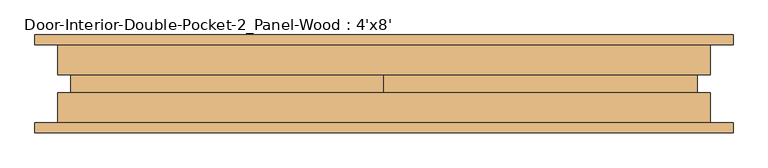
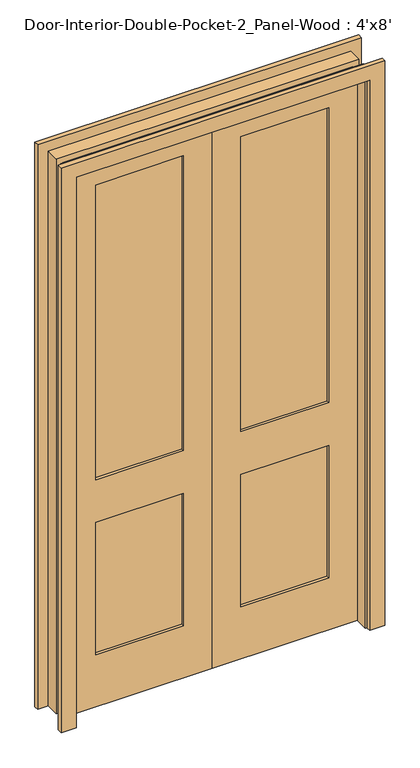
"""IFC4 building model written with IfcOpenShell, lengths in millimetres: door geometry, Door-Interior-Double-Pocket-2_Panel-Wood : 4'x8'."""

from ifc_helpers import new_model, si_unit, frame, origin, place, context, project, spatial, polyline, outline, extrude, source, transform, mapped, element, save


def door_interior_double_pocket_2_panel_wood_4_x8_0aea24c3(model_context):
    return source(origin(), model_context, "Body", "SweptSolid", [
        extrude(outline(polyline([(0.0, 615.95), (0.0, 679.45), (2508.25, 679.45), (2508.25, -679.45), (0.0, -679.45), (0.0, -615.95), (2444.75, -615.95), (2444.75, 615.95), (0.0, 615.95)])), frame((0.0, 76.2, 0.0), z_axis=(0.0, 1.0, 0.0), x_axis=(0.0, 0.0, 1.0)), (0.0, 0.0, 1.0), 19.05),
        extrude(outline(polyline([(0.0, 615.95), (0.0, 679.45), (2508.25, 679.45), (2508.25, -679.45), (0.0, -679.45), (0.0, -615.95), (2444.75, -615.95), (2444.75, 615.95), (0.0, 615.95)])), frame((0.0, -95.25, 0.0), z_axis=(0.0, 1.0, 0.0), x_axis=(0.0, 0.0, 1.0)), (0.0, 0.0, 1.0), 19.05),
        extrude(outline(polyline([(2438.4, 0.0), (0.0, 0.0), (0.0, 609.6), (2438.4, 609.6), (2438.4, 0.0)]), holes=[polyline([(2319.3375, 120.65), (2319.3375, 488.95), (1009.65, 488.95), (1009.65, 120.65), (2319.3375, 120.65)]), polyline([(819.15, 120.65), (819.15, 488.95), (231.775, 488.95), (231.775, 120.65), (819.15, 120.65)])]), frame((0.0, -17.4625, 0.0), z_axis=(0.0, 1.0, 0.0), x_axis=(0.0, 0.0, 1.0)), (0.0, 0.0, 1.0), 34.925),
        extrude(outline(polyline([(488.95, -5.8208333), (120.65, -5.8208333), (120.65, 5.8208333), (488.95, 5.8208333), (488.95, -5.8208333)])), frame((0.0, 0.0, 1009.65), z_axis=(0.0, 0.0, 1.0), x_axis=(1.0, 0.0, 0.0)), (0.0, 0.0, 1.0), 1309.6875),
        extrude(outline(polyline([(488.95, -5.8208333), (120.65, -5.8208333), (120.65, 5.8208333), (488.95, 5.8208333), (488.95, -5.8208333)])), frame((0.0, 0.0, 231.775), z_axis=(0.0, 0.0, 1.0), x_axis=(1.0, 0.0, 0.0)), (0.0, 0.0, 1.0), 587.375),
        extrude(outline(polyline([(0.0, 635.0), (2463.8, 635.0), (2463.8, -635.0), (0.0, -635.0), (0.0, -609.6), (2438.4, -609.6), (2438.4, 609.6), (0.0, 609.6), (0.0, 635.0)])), frame((0.0, 17.4625, 0.0), z_axis=(0.0, 1.0, 0.0), x_axis=(0.0, 0.0, 1.0)), (0.0, 0.0, 1.0), 58.7375),
        extrude(outline(polyline([(0.0, 635.0), (2463.8, 635.0), (2463.8, -635.0), (0.0, -635.0), (0.0, -609.6), (2438.4, -609.6), (2438.4, 609.6), (0.0, 609.6), (0.0, 635.0)])), frame((0.0, -76.2, 0.0), z_axis=(0.0, 1.0, 0.0), x_axis=(0.0, 0.0, 1.0)), (0.0, 0.0, 1.0), 58.7375),
        extrude(outline(polyline([(2438.4, -609.6), (0.0, -609.6), (0.0, 0.0), (2438.4, 0.0), (2438.4, -609.6)]), holes=[polyline([(2319.3375, -488.95), (2319.3375, -120.65), (1009.65, -120.65), (1009.65, -488.95), (2319.3375, -488.95)]), polyline([(819.15, -488.95), (819.15, -120.65), (231.775, -120.65), (231.775, -488.95), (819.15, -488.95)])]), frame((0.0, -17.4625, 0.0), z_axis=(0.0, 1.0, 0.0), x_axis=(0.0, 0.0, 1.0)), (0.0, 0.0, 1.0), 34.925),
        extrude(outline(polyline([(-120.65, -5.8208333), (-488.95, -5.8208333), (-488.95, 5.8208333), (-120.65, 5.8208333), (-120.65, -5.8208333)])), frame((0.0, 0.0, 1009.65), z_axis=(0.0, 0.0, 1.0), x_axis=(1.0, 0.0, 0.0)), (0.0, 0.0, 1.0), 1309.6875),
        extrude(outline(polyline([(-120.65, -5.8208333), (-488.95, -5.8208333), (-488.95, 5.8208333), (-120.65, 5.8208333), (-120.65, -5.8208333)])), frame((0.0, 0.0, 231.775), z_axis=(0.0, 0.0, 1.0), x_axis=(1.0, 0.0, 0.0)), (0.0, 0.0, 1.0), 587.375),
    ])


if __name__ == "__main__":
    model = new_model("IFC4")
    model_context = context("Model", 3, world=origin())
    ifc_project = project(units=[si_unit("LENGTHUNIT", "METRE", prefix="MILLI")], contexts=[model_context])
    site = spatial("IfcSite", under=ifc_project)
    building = spatial("IfcBuilding", under=site)
    placement = place(None, origin())
    door_interior_double_pocket_2_panel_wood_4_x8_shape = door_interior_double_pocket_2_panel_wood_4_x8_0aea24c3(model_context)
    element("IfcDoor", 1, ObjectType="Door-Interior-Double-Pocket-2_Panel-Wood : 4'x8'", at=placement, inside=building, context=model_context, shape_type="MappedRepresentation", body=[
        mapped(door_interior_double_pocket_2_panel_wood_4_x8_shape, transform((0.0, 0.0, 0.0), x_axis=(1.0, 0.0, 0.0), y_axis=(0.0, 1.0, 0.0), z_axis=(0.0, 0.0, 1.0))),
    ])
    save(model, "model.ifc")

# Revit data of these elements
# Type "Door-Interior-Double-Pocket-2_Panel-Wood : 4'x8'"
#   Type Mark = "11"
#   Assembly Code = "C1020300"
#   Analytic Construction = "Wooden"
#   Top Rail = 0' - 4 11/16"
#   Thickness = 0' - 1 3/8"
#   Thermal Resistance (R) = 2.5876 (h·ft²·°F)/BTU
#   Stiles = 0' - 4 3/4"
#   Rough Width = 8' - 2"
#   Rough Height = 8' - 4 1/2"
#   Panel Width = 2' - 0"
#   Lock Rail = 0' - 7 1/2"
#   Location [instance default] = 2' - 1"
#   Height = 8' - 0"
#   Width = 4' - 0"
#   Heat Transfer Coefficient (U) = 0.3865 BTU/(h·ft²·°F)
#   Bottom Rail = 0' - 9 1/8"
#   Panel Open [instance default] = no
#   Trim Material = Cherry
#   Panel Material = Cherry
#   Frame Material = Cherry
#   Visual Light Transmittance = 0
#   Solar Heat Gain Coefficient = 0
#   Wall Closure = (empty or 0)
#   Function = (empty or 0)
# Element 1 (IfcDoor, "Door-Interior-Double-Pocket-2_Panel-Wood : 4'x8'")
#   Materials on its faces: "Cherry"
# Materials
#   "Cherry": class "Wood", colour RGB 226 177 128, transparency 0, Description = "Prunus Serotina", Cost = 0
